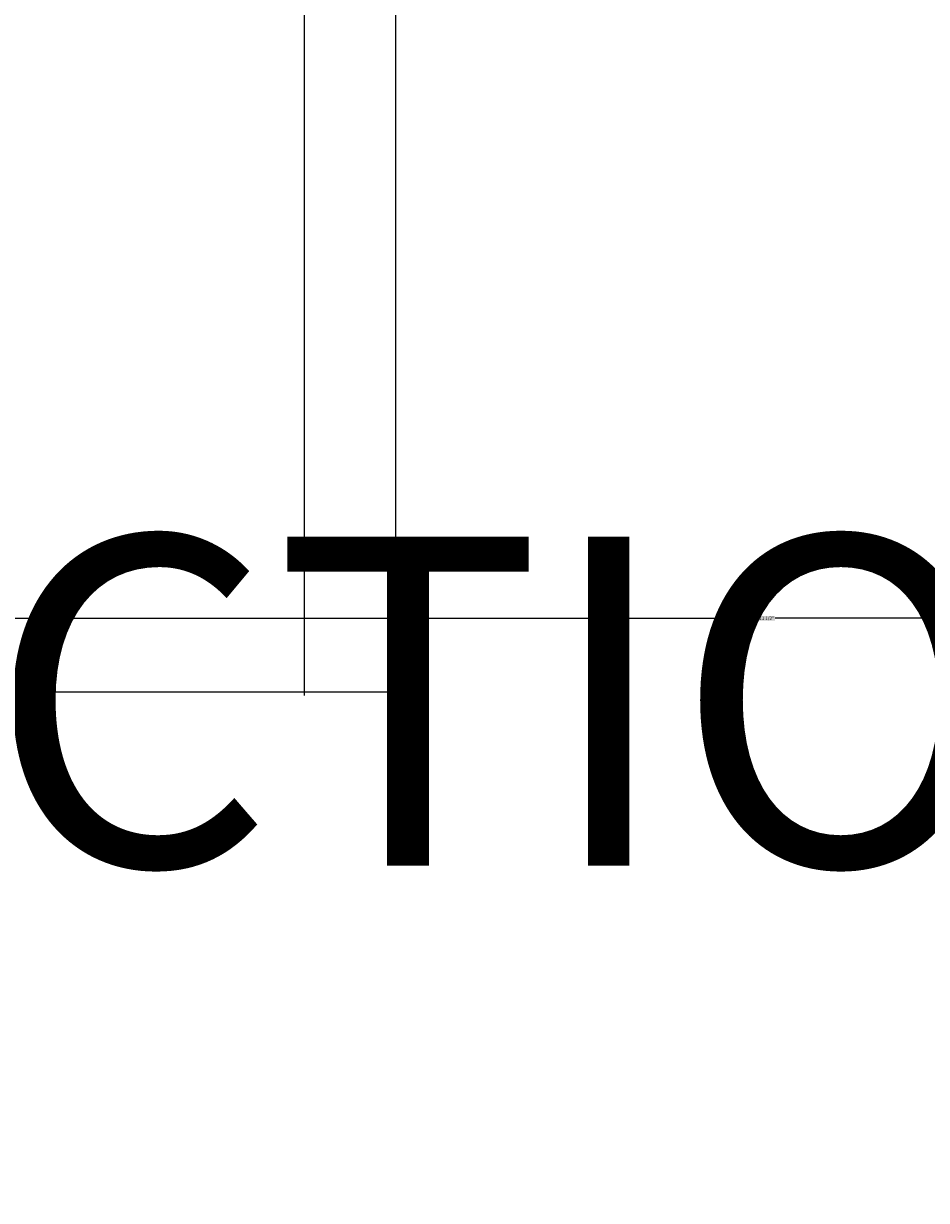
# Model space of a CAD drawing. Units: inches. Extents: x -301 to 715, y -607 to 364.
# Tile 43 of 141: x -66 to -17, y -324 to -260. Entities that reach past the tile are written whole.
import ezdxf

# ---------------------------------------------------------------- set-up
doc = ezdxf.new("R2010")
doc.units = ezdxf.units.IN
doc.header["$MEASUREMENT"] = 0
doc.layers.add('A-ANNO-DIMS', color=2, linetype='Continuous', lineweight=18)
doc.layers.add('A-ANNO-TITL', color=1, linetype='Continuous', lineweight=35)
doc.styles.get("Standard").update_dxf_attribs({"font": 'arial.ttf'})
doc.dimstyles.get("Standard").update_dxf_attribs({"dimtxt": 0.18, "dimasz": 0.18, "dimexe": 0.18, "dimexo": 0.0625, "dimgap": 0.09, "dimtad": 0, "dimtih": 1, "dimtoh": 1, "dimdec": 1, "dimzin": 0, "dimdsep": 46, "dimlunit": 4, "dimtxsty": 'Standard', "dimcen": 0.09, "dimclrd": 3, "dimclre": 4, "dimclrt": 6, "dimadec": 0, "dimazin": 0, "dimtfac": 1, "dimtdec": 1, "dimtofl": 0, "dimtmove": 0, "dimatfit": 3, "dimfxl": 1, "dimtfill": 2, "dimtfillclr": 51, "dimtolj": 1, "dimtzin": 0, "dimarcsym": 0})

# ---------------------------------------------------------------- blocks, each defined once
blk = doc.blocks.new('*D147')
at = {"layer": 'A-ANNO-DIMS', "color": 4, "lineweight": -2, "transparency": 16777216}
for p, q in [((-103.603, -223.88), (-103.603, -296.865)), ((-45.603, -223.88), (-45.603, -296.865))]:
    blk.add_line(p, q, dxfattribs=at)
at = {"layer": 'A-ANNO-DIMS', "color": 3, "lineweight": -2, "transparency": 16777216}
for p, q in [((-103.423, -296.685), (-75.006, -296.685)), ((-45.783, -296.685), (-74.2, -296.685))]:
    blk.add_line(p, q, dxfattribs=at)
at = {"layer": 'A-ANNO-DIMS', "color": 3, "transparency": 16777216}
for points in [[(-103.423, -296.655), (-103.423, -296.715), (-103.603, -296.685)], [(-45.783, -296.655), (-45.783, -296.715), (-45.603, -296.685)]]:
    blk.add_solid(points, dxfattribs=at)
at = {"layer": 'Defpoints', "color": 0, "transparency": 16777216}
for p in [(-103.603, -223.818), (-45.603, -223.818), (-45.603, -296.685)]:
    blk.add_point(p, dxfattribs=at)
at = {"layer": 'A-ANNO-DIMS', "color": 6, "transparency": 16777216, "insert": (-74.603, -296.685), "char_height": 0.18, "attachment_point": 5, "bg_fill": 1, "box_fill_scale": 1.25, "bg_fill_color": 51, "bg_fill_transparency": 0}
blk.add_mtext('\\A1;4\'-10"', dxfattribs=at)
blk = doc.blocks.new('*D158')
at = {"layer": 'A-ANNO-DIMS', "color": 4, "lineweight": -2, "transparency": 16777216}
for p, q in [((-122.603, 221.62), (-122.603, -296.865)), ((-50.603, 221.62), (-50.603, -296.865))]:
    blk.add_line(p, q, dxfattribs=at)
at = {"layer": 'A-ANNO-DIMS', "color": 3, "lineweight": -2, "transparency": 16777216}
for p, q in [((-122.423, -296.685), (-86.933, -296.685)), ((-50.783, -296.685), (-86.274, -296.685))]:
    blk.add_line(p, q, dxfattribs=at)
at = {"layer": 'A-ANNO-DIMS', "color": 3, "transparency": 16777216}
for points in [[(-122.423, -296.655), (-122.423, -296.715), (-122.603, -296.685)], [(-50.783, -296.655), (-50.783, -296.715), (-50.603, -296.685)]]:
    blk.add_solid(points, dxfattribs=at)
at = {"layer": 'Defpoints', "color": 0, "transparency": 16777216}
for p in [(-122.603, 221.682), (-50.603, 221.682), (-50.603, -296.685)]:
    blk.add_point(p, dxfattribs=at)
at = {"layer": 'A-ANNO-DIMS', "color": 6, "transparency": 16777216, "insert": (-86.603, -296.685), "char_height": 0.18, "attachment_point": 5, "bg_fill": 1, "box_fill_scale": 1.25, "bg_fill_color": 51, "bg_fill_transparency": 0}
blk.add_mtext('\\A1;6\'-0"', dxfattribs=at)
blk = doc.blocks.new('*D175')
at = {"layer": 'A-ANNO-DIMS', "color": 4, "lineweight": -2, "transparency": 16777216}
for p, q in [((-199.282, -324.415), (-199.282, -292.467)), ((148.218, -324.415), (148.218, -292.467))]:
    blk.add_line(p, q, dxfattribs=at)
at = {"layer": 'A-ANNO-DIMS', "color": 3, "lineweight": -2, "transparency": 16777216}
for p, q in [((-199.102, -292.647), (-26.212, -292.647)), ((148.038, -292.647), (-24.852, -292.647))]:
    blk.add_line(p, q, dxfattribs=at)
at = {"layer": 'A-ANNO-DIMS', "color": 3, "transparency": 16777216}
for points in [[(-199.102, -292.617), (-199.102, -292.677), (-199.282, -292.647)], [(148.038, -292.617), (148.038, -292.677), (148.218, -292.647)]]:
    blk.add_solid(points, dxfattribs=at)
at = {"layer": 'Defpoints', "color": 0, "transparency": 16777216}
for p in [(148.218, -292.647), (-199.282, -324.477), (148.218, -324.477)]:
    blk.add_point(p, dxfattribs=at)
at = {"layer": 'A-ANNO-DIMS', "color": 6, "transparency": 16777216, "insert": (-25.532, -292.647), "char_height": 0.18, "attachment_point": 5, "bg_fill": 1, "box_fill_scale": 1.25, "bg_fill_color": 51, "bg_fill_transparency": 0}
blk.add_mtext('\\A1;28\'-11 1/2"', dxfattribs=at)

msp = doc.modelspace()

# ---------------------------------------------------------------- texts
at = {"layer": 'A-ANNO-TITL'}
msp.add_text('SECTION', height=18, dxfattribs=at).set_placement((-97.05, -306.177))

# ---------------------------------------------------------------- dimensions: what is measured, and where the dimension line sits
at = {"layer": 'A-ANNO-DIMS'}
for base, p1, p2, picture, middle in [((-50.603, -296.685), (-122.603, 221.682), (-50.603, 221.682), '*D158', (-86.603, -296.685)), ((-45.603, -296.685), (-103.603, -223.818), (-45.603, -223.818), '*D147', (-74.603, -296.685)), ((148.218, -292.647), (-199.282, -324.477), (148.218, -324.477), '*D175', (-25.532, -292.647))]:
    dim = msp.add_linear_dim(base=base, p1=p1, p2=p2, dimstyle='Standard', override={"dimdec": 1, "dimlfac": 1, "dimrnd": 0, "dimzin": 1, "dimdsep": 46, "dimlunit": 4, "dimfrac": 2}, dxfattribs=at)
    dim.commit()
    dim.dimension.update_dxf_attribs({"geometry": picture, "text_midpoint": middle})

doc.saveas('drawing.dxf')
